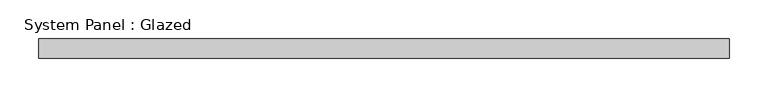
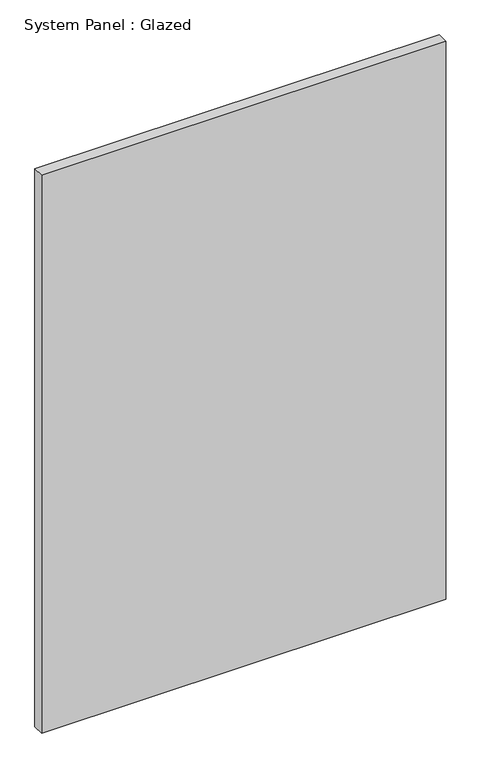
"""IFC4 building model written with IfcOpenShell, lengths in millimetres: plate geometry, System Panel : Glazed."""

from ifc_helpers import new_model, si_unit, origin, origin_with_axes, place, context, project, spatial, polyline, outline, extrude, source, transform, mapped, element, save


def system_panel_glazed_88eb0887(model_context):
    return source(origin(), model_context, "Body", "SweptSolid", [
        extrude(outline(polyline([(447.675, 19.05), (-447.675, 19.05), (-447.675, 44.45), (447.675, 44.45), (447.675, 19.05)])), origin_with_axes(), (0.0, 0.0, 1.0), 1305.9498103),
    ])


if __name__ == "__main__":
    model = new_model("IFC4")
    model_context = context("Model", 3, world=origin())
    ifc_project = project(units=[si_unit("LENGTHUNIT", "METRE", prefix="MILLI")], contexts=[model_context])
    site = spatial("IfcSite", under=ifc_project)
    building = spatial("IfcBuilding", under=site)
    placement = place(None, origin())
    system_panel_glazed_shape = system_panel_glazed_88eb0887(model_context)
    element("IfcPlate", 1, ObjectType="System Panel : Glazed", at=placement, inside=building, context=model_context, shape_type="MappedRepresentation", body=[
        mapped(system_panel_glazed_shape, transform((0.0, 0.0, 0.0), x_axis=(1.0, 0.0, 0.0), y_axis=(0.0, 1.0, 0.0), z_axis=(0.0, 0.0, 1.0))),
    ])
    save(model, "model.ifc")

# Revit data of these elements
# Type "System Panel : Glazed"
#   Construction Type Id = "GSP4R"
#   Analytic Construction = "1/8 in Pilkington single glazing"
#   Visual Light Transmittance = 0.9
#   Solar Heat Gain Coefficient = 0.86
#   Heat Transfer Coefficient (U) = 1.18115 BTU/(h·ft²·°F)
#   Define Thermal Properties by = 1
# Element 1 (IfcPlate, "System Panel : Glazed")
#   Materials on its faces: "Glass"
# Materials
#   "Glass": class "Glass", colour RGB 0 128 192, transparency 0.75, Description = "Soda Lime Glass", Cost = 0
